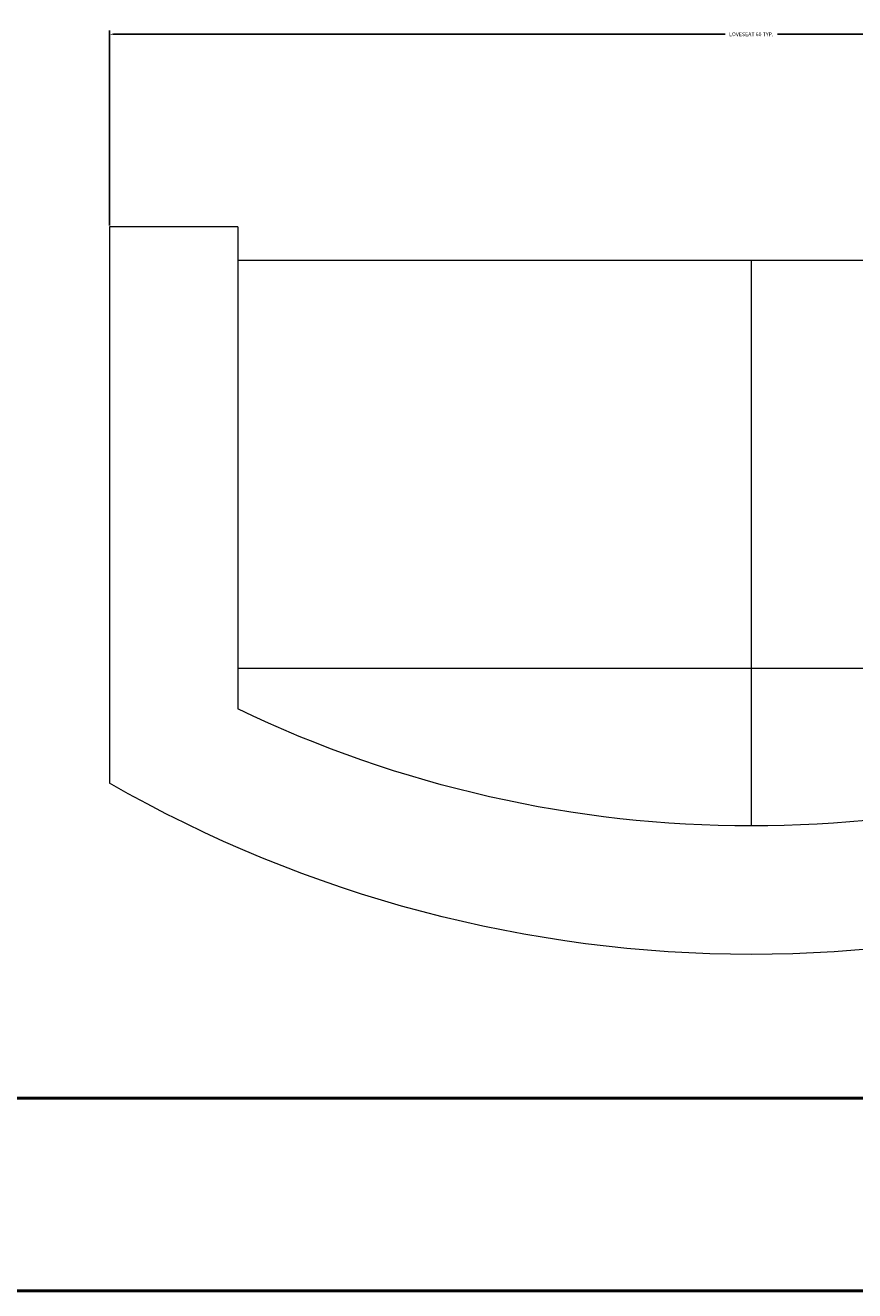
# Model space of a CAD drawing. Units: inches. Extents: x 7359 to 7979, y 33027 to 34263.
# Tile 22 of 32: x 7511 to 7550, y 33765 to 33824. Entities that reach past the tile are written whole.
import ezdxf

# ---------------------------------------------------------------- set-up
doc = ezdxf.new("R2010")
doc.units = ezdxf.units.IN
for name, color, linetype, lineweight in [('A-ANNO-DIMS', 2, 'Continuous', 18), ('A-FURN', 8, 'Continuous', 18), ('A-WALL', 7, 'Continuous', 50)]:
    doc.layers.add(name, color=color, linetype=linetype, lineweight=lineweight)
doc.styles.get("Standard").update_dxf_attribs({"font": 'arial.ttf'})
doc.dimstyles.get("Standard").update_dxf_attribs({"dimtxt": 0.18, "dimasz": 0.18, "dimexe": 0.18, "dimexo": 0.0625, "dimgap": 0.09, "dimtad": 0, "dimtih": 1, "dimtoh": 1, "dimdec": 4, "dimzin": 0, "dimdsep": 46, "dimtxsty": 'Standard', "dimcen": 0.09, "dimadec": 0, "dimazin": 0, "dimtfac": 1, "dimtdec": 4, "dimtofl": 0, "dimtmove": 0, "dimatfit": 3, "dimfxl": 1, "dimtolj": 1, "dimtzin": 0, "dimarcsym": 0})

# ---------------------------------------------------------------- blocks, each defined once
blk = doc.blocks.new('Sofa - Roundback Loveseat 5 ft.')
for p, q in [((0, -32.44198), (0, -5.99998)), ((-24, -33.99998), (-24, -11.46958)), ((24.00004, -33.99998), (24.00004, -11.46958)), ((-23.9998, -13.38178), (23.99986, -13.38178)), ((-24, -32.44198), (24.00004, -32.44198))]:
    blk.add_line(p, q)
for points in [[(-24, -33.99998), (-30, -33.99998), (-30, -7.99998)], [(30.00004, -7.99998), (30.00004, -33.99998), (24.00004, -33.99998)]]:
    blk.add_lwpolyline(points)
for centre, radius, start, end in [((0, -60.24998), 60.24998, 60.13715, 119.8628), ((0, -61.38438), 55.38444, 64.32083, 115.6792)]:
    blk.add_arc(centre, radius, start, end)
blk = doc.blocks.new('*D26')
at = {"layer": 'A-ANNO-DIMS', "color": 0, "lineweight": -2, "transparency": 16777216}
for p, q in [((7515.397, 33814.613), (7515.397, 33823.731)), ((7515.577, 33823.551), (7544.174, 33823.551)), ((7575.217, 33823.551), (7546.62, 33823.551)), ((7575.397, 33814.613), (7575.397, 33823.731))]:
    blk.add_line(p, q, dxfattribs=at)
at = {"layer": 'A-ANNO-DIMS', "color": 0, "transparency": 16777216}
for points in [[(7515.577, 33823.581), (7515.577, 33823.521), (7515.397, 33823.551)], [(7575.217, 33823.581), (7575.217, 33823.521), (7575.397, 33823.551)]]:
    blk.add_solid(points, dxfattribs=at)
at = {"layer": 'Defpoints', "color": 0, "transparency": 16777216}
for p in [(7575.397, 33823.551), (7515.397, 33814.551), (7575.397, 33814.551)]:
    blk.add_point(p, dxfattribs=at)
at = {"layer": 'A-ANNO-DIMS', "color": 0, "transparency": 16777216, "insert": (7545.397, 33823.551), "char_height": 0.18, "attachment_point": 5}
blk.add_mtext('\\A1;LOVESEAT 60 TYP.', dxfattribs=at)

msp = doc.modelspace()

# ---------------------------------------------------------------- linework, layer by layer
at = {"layer": 'A-WALL'}
for p, q in [((7467.5915, 33773.8339), (7689.4915, 33773.8339)), ((7458.5915, 33764.8339), (7883.9915, 33764.8339))]:
    msp.add_line(p, q, dxfattribs=at)

# ---------------------------------------------------------------- block references
at = {"layer": 'A-FURN', "xscale": -1, "rotation": 180}
msp.add_blockref('Sofa - Roundback Loveseat 5 ft.', (7545.3969, 33780.551), dxfattribs=at)

# ---------------------------------------------------------------- dimensions: what is measured, and where the dimension line sits
at = {"layer": 'A-ANNO-DIMS'}
dim = msp.add_linear_dim(base=(7575.397, 33823.551), p1=(7515.3969, 33814.551), p2=(7575.397, 33814.551), text='LOVESEAT <> TYP.', dimstyle='Standard', override={"dimdec": 0, "dimlfac": 1, "dimrnd": 0, "dimzin": 0, "dimdsep": 46, "dimlunit": 2}, dxfattribs=at)
dim.commit()
dim.dimension.update_dxf_attribs({"geometry": '*D26', "text_midpoint": (7545.397, 33823.551)})

doc.saveas('drawing.dxf')
